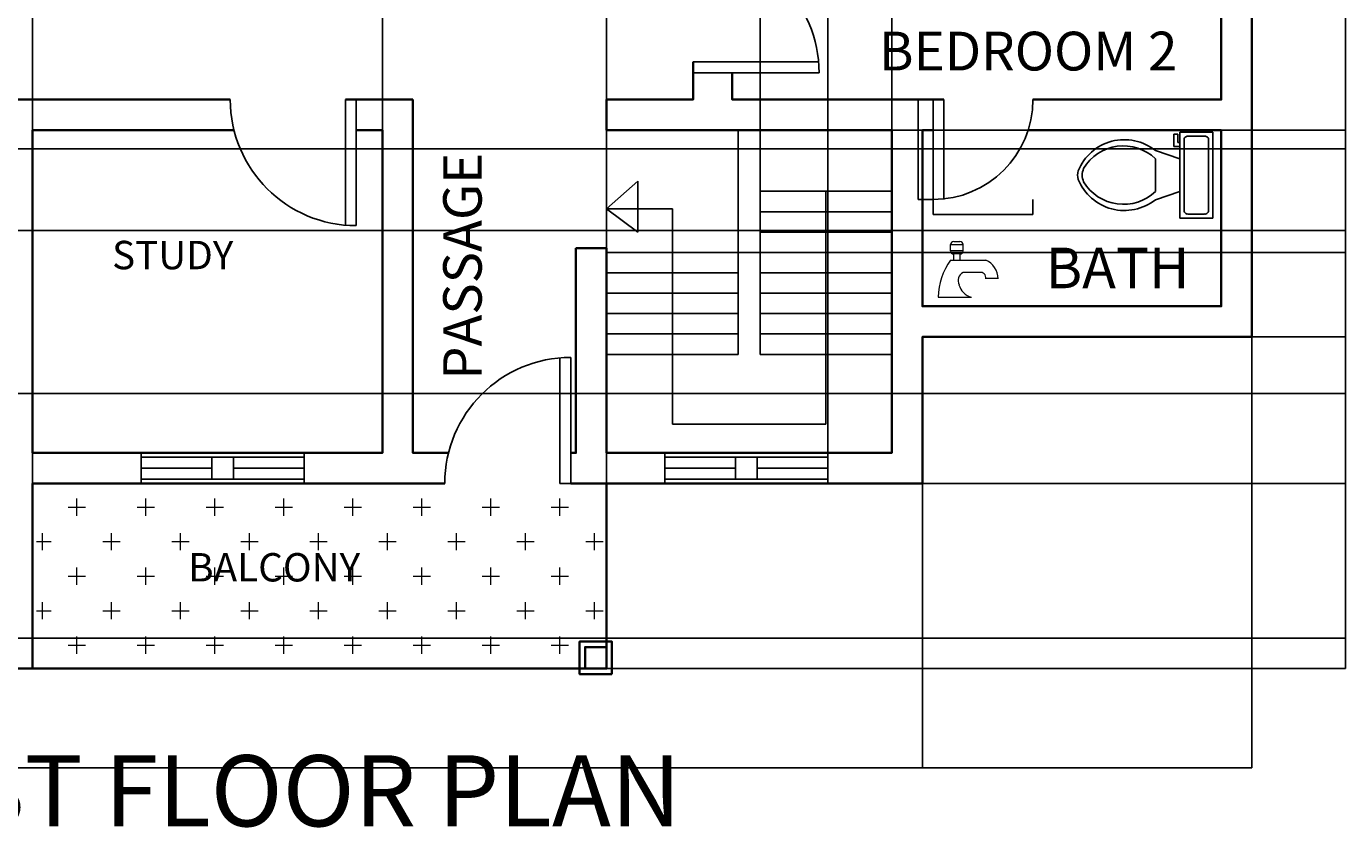
# Model space of a CAD drawing. Units: millimetres. Extents: x 19292 to 100733, y 12374 to 26974.
# Tile 20 of 24: x 47819 to 57530, y 12374 to 18270. Entities that reach past the tile are written whole.
import ezdxf

# ---------------------------------------------------------------- set-up
doc = ezdxf.new("R2010")
doc.units = ezdxf.units.MM
for name, color, linetype, lineweight in [('A-ANNO-DIMS', 2, 'Continuous', 18), ('A-ANNO-TEXT', 7, 'Continuous', 35), ('A-AREA-IDEN', 3, 'Continuous', 25), ('A-DOOR', 4, 'Continuous', 25), ('A-FLOR-FIXT', 9, 'Continuous', 18), ('A-FLOR-PATT', 252, 'Continuous', 13), ('A-FLOR-STRS', 1, 'Continuous', 25), ('A-GLAZ', 3, 'Continuous', 25), ('A-WALL', 7, 'Continuous', 35)]:
    doc.layers.add(name, color=color, linetype=linetype, lineweight=lineweight)
doc.layers.add('FURNITURE', color=40, linetype='Continuous')
doc.layers.add('WINDOWS', color=50, linetype='Continuous')
doc.styles.get("Standard").update_dxf_attribs({"font": 'arial.ttf'})
doc.dimstyles.get("Standard").update_dxf_attribs({"dimtxt": 0.18, "dimasz": 0.18, "dimexe": 0.18, "dimexo": 0.0625, "dimgap": 0.09, "dimtad": 0, "dimtih": 1, "dimtoh": 1, "dimdec": 4, "dimzin": 0, "dimdsep": 46, "dimtxsty": 'Standard', "dimcen": 0.09, "dimadec": 0, "dimazin": 0, "dimtfac": 1, "dimtdec": 4, "dimtofl": 0, "dimtmove": 0, "dimatfit": 3, "dimfxl": 1, "dimtolj": 1, "dimtzin": 0, "dimarcsym": 0})

# ---------------------------------------------------------------- blocks, each defined once
blk = doc.blocks.new('WW')
at = {"layer": 'WINDOWS'}
for p, q in [((-5183.9, -4940.9), (-3983.9, -4940.9)), ((-4663.9, -4940.9), (-4663.9, -5100.9)), ((-4503.9, -4940.9), (-4503.9, -5100.9)), ((-4503.9, -4940.9), (-4503.9, -5100.9)), ((-5183.9, -5020.9), (-4663.9, -5020.9)), ((-4503.9, -5020.9), (-3983.9, -5020.9)), ((-5183.9, -5100.9), (-3983.9, -5100.9))]:
    blk.add_line(p, q, dxfattribs=at)
for points in [[(-5183.9, -5133.4), (-5183.9, -4908.4)], [(-3983.9, -4908.4), (-3983.9, -5133.4)]]:
    blk.add_lwpolyline(points, dxfattribs=at)
blk = doc.blocks.new('WC01')
at = {"layer": 'FURNITURE'}
for p, q in [((10.5, 0), (-10.5, 0)), ((-10.5, 0), (-10.5, -8)), ((10.5, -8), (10.5, 0)), ((-9.5, -2), (-9.5, -6)), ((8.5, -1), (-8.5, -1)), ((9.5, -6), (9.5, -2)), ((-10.5, -8), (10.5, -8)), ((-10, -9.5), (-10, -8.5)), ((-10, -8.5), (-8, -8.5)), ((-7, -9.5), (-10, -9.5)), ((-8.5, -7), (8.5, -7)), ((-8, -8.5), (-8, -8)), ((-7, -8), (-7, -9.5)), ((-4, -8), (-6, -14)), ((4, -8), (6, -14)), ((4, -14), (-4, -14))]:
    blk.add_line(p, q, dxfattribs=at)
for centre, radius, start, end in [((-8.62, -1.88), 0.884, 81.8699, 188.1301), ((8.62, -1.88), 0.884, 351.8699, 98.1301), ((-8.62, -6.12), 0.884, 171.8699, 278.1301), ((8.62, -6.12), 0.884, 261.8699, 8.1301), ((3.52, -21.58), 12.17, 141.4691, 247.9714), ((4.2, -21.82), 11.33, 136.3677, 238.9468), ((-3.52, -21.58), 12.17, 292.0284, 38.5307), ((-4.2, -21.82), 11.33, 301.053, 43.6321), ((0, -27.88), 4, 245.7318, 294.2682), ((0, -29), 4, 254.8605, 285.1395)]:
    blk.add_arc(centre, radius, start, end, dxfattribs=at)
blk = doc.blocks.new('TAP-SIDELEV')
for p, q in [((1, 4.25), (2, 4.25)), ((2, 3.75), (1, 3.75)), ((1.25, 3), (1.25, 3.5)), ((1.75, 3.5), (1.75, 3)), ((1, 3), (3.84, 3)), ((3.53, 2), (2, 2)), ((4.84, 1.5), (3.84, 1.5)), ((0, 0), (0.25, 0)), ((0.25, 0), (2.68, 0))]:
    blk.add_line(p, q)
for points in [[(1.25, 4.5), (1.75, 4.5)], [(1, 3.75), (1, 4.25)], [(1.75, 3.5), (1.25, 3.5)], [(2, 4.25), (2, 3.75)]]:
    blk.add_lwpolyline(points)
for centre, radius, start, end in [((1.24, 4.26), 0.243, 88.2224, 181.7776), ((1.76, 4.26), 0.243, 358.2224, 91.7776), ((1.24, 3.74), 0.243, 178.2224, 271.7776), ((1.76, 3.74), 0.243, 268.2224, 1.7776), ((5.08, -0.03), 5.08, 143.4467, 179.6834), ((3.17, 1.47), 1.67, 0.9828, 66.4049), ((2.38, 1.33), 0.773, 119.1801, 204.8716), ((3.43, 1.59), 0.417, 347.0192, 102.9808), ((3.05, 1.38), 1.43, 195.2551, 254.7449)]:
    blk.add_arc(centre, radius, start, end)
blk = doc.blocks.new('DOOR-900')
for p, q in [((927.7, 80), (0, 80)), ((927.7, 0), (927.7, 80)), ((927.7, 0), (927.7, 80)), ((927.7, 0), (0, 0))]:
    blk.add_line(p, q)
blk.add_arc((927.7, 0), 927.7, 90, 180)
blk = doc.blocks.new('DOOR-SWING-900')
blk.add_line((927.7, 927.7), (927.7, 0))
blk.add_arc((927.7, 927.7), 927.7, 180, 270)
blk = doc.blocks.new('DOOR-SWING-750')
blk.add_line((0, 0), (735.3, 0))
blk.add_arc((0, 0), 735.3, 0, 90)
blk = doc.blocks.new('*D32')
at = {"layer": 'A-ANNO-DIMS', "color": 0, "lineweight": -2, "transparency": 16777216}
for p, q in [((54493.3, 16996.1), (54493.3, 16885.7)), ((55228.6, 16996.1), (55228.6, 16885.7)), ((54493.5, 16885.8), (54859.7, 16885.8)), ((55228.4, 16885.8), (54862.2, 16885.8))]:
    blk.add_line(p, q, dxfattribs=at)
at = {"layer": 'A-ANNO-DIMS', "color": 0, "transparency": 16777216}
for points in [[(54493.5, 16885.9), (54493.5, 16885.8), (54493.3, 16885.8)], [(55228.4, 16885.9), (55228.4, 16885.8), (55228.6, 16885.8)]]:
    blk.add_solid(points, dxfattribs=at)
at = {"layer": 'Defpoints', "color": 0, "transparency": 16777216}
for p in [(54493.3, 16996.1), (55228.6, 16996.1), (55228.6, 16885.8)]:
    blk.add_point(p, dxfattribs=at)
at = {"layer": 'A-ANNO-DIMS', "color": 0, "transparency": 16777216, "insert": (54860.9, 16885.8), "char_height": 0.18, "attachment_point": 5}
blk.add_mtext('\\A1;DOOR 750 735 TYP.', dxfattribs=at)
blk = doc.blocks.new('*D33')
at = {"layer": 'A-ANNO-DIMS', "color": 0, "lineweight": -2, "transparency": 16777216}
for p, q in [((54493.2, 17731.4), (54382.8, 17731.4)), ((54383, 17731.2), (54383, 17363.9)), ((54383, 16996.3), (54383, 17363.6)), ((54493.2, 16996.1), (54382.8, 16996.1))]:
    blk.add_line(p, q, dxfattribs=at)
at = {"layer": 'A-ANNO-DIMS', "color": 0, "transparency": 16777216}
for points in [[(54383, 17731.2), (54383, 17731.2), (54383, 17731.4)], [(54383, 16996.3), (54383, 16996.3), (54383, 16996.1)]]:
    blk.add_solid(points, dxfattribs=at)
at = {"layer": 'Defpoints', "color": 0, "transparency": 16777216}
for p in [(54493.3, 17731.4), (54383, 16996.1), (54493.3, 16996.1)]:
    blk.add_point(p, dxfattribs=at)
at = {"layer": 'A-ANNO-DIMS', "color": 0, "transparency": 16777216, "insert": (54383, 17363.8), "char_height": 0.18, "attachment_point": 5}
blk.add_mtext('\\A1;735 TYP.', dxfattribs=at)
blk = doc.blocks.new('*D103')
at = {"layer": 'A-ANNO-DIMS', "color": 0, "lineweight": -2, "transparency": 16777216}
for p, q in [((44268, 15569), (57530.2, 15569)), ((57530, 15568.8), (57530, 14669.2)), ((57530, 13769.2), (57530, 14668.8)), ((44268, 13769), (57530.2, 13769))]:
    blk.add_line(p, q, dxfattribs=at)
at = {"layer": 'A-ANNO-DIMS', "color": 0, "transparency": 16777216}
for points in [[(57530, 15568.8), (57530.1, 15568.8), (57530, 15569)], [(57530, 13769.2), (57530.1, 13769.2), (57530, 13769)]]:
    blk.add_solid(points, dxfattribs=at)
at = {"layer": 'Defpoints', "color": 0, "transparency": 16777216}
for p in [(44268, 15569), (57530, 15569), (44268, 13769)]:
    blk.add_point(p, dxfattribs=at)
at = {"layer": 'A-ANNO-DIMS', "color": 0, "transparency": 16777216, "insert": (57530, 14669), "char_height": 0.18, "attachment_point": 5}
blk.add_mtext('\\A1;1800', dxfattribs=at)
blk = doc.blocks.new('*D104')
at = {"layer": 'A-ANNO-DIMS', "color": 0, "lineweight": -2, "transparency": 16777216}
for p, q in [((44268, 17369), (57530.2, 17369)), ((57530, 17368.8), (57530, 17069.2)), ((57530, 16769.2), (57530, 17068.8)), ((44268, 16769), (57530.2, 16769))]:
    blk.add_line(p, q, dxfattribs=at)
at = {"layer": 'A-ANNO-DIMS', "color": 0, "transparency": 16777216}
for points in [[(57530, 17368.8), (57530.1, 17368.8), (57530, 17369)], [(57530, 16769.2), (57530.1, 16769.2), (57530, 16769)]]:
    blk.add_solid(points, dxfattribs=at)
at = {"layer": 'Defpoints', "color": 0, "transparency": 16777216}
for p in [(44268, 17369), (57530, 17369), (44268, 16769)]:
    blk.add_point(p, dxfattribs=at)
at = {"layer": 'A-ANNO-DIMS', "color": 0, "transparency": 16777216, "insert": (57530, 17069), "char_height": 0.18, "attachment_point": 5}
blk.add_mtext('\\A1;600', dxfattribs=at)
blk = doc.blocks.new('*D105')
at = {"layer": 'A-ANNO-DIMS', "color": 0, "lineweight": -2, "transparency": 16777216}
for p, q in [((54414.6, 14906.4), (57530.2, 14906.4)), ((57530, 14906.2), (57530, 14225.4)), ((57530, 13544.2), (57530, 14225)), ((52089.7, 13544), (57530.2, 13544))]:
    blk.add_line(p, q, dxfattribs=at)
at = {"layer": 'A-ANNO-DIMS', "color": 0, "transparency": 16777216}
for points in [[(57530, 14906.2), (57530.1, 14906.2), (57530, 14906.4)], [(57530, 13544.2), (57530.1, 13544.2), (57530, 13544)]]:
    blk.add_solid(points, dxfattribs=at)
at = {"layer": 'Defpoints', "color": 0, "transparency": 16777216}
for p in [(54414.5, 14906.4), (57530, 14906.4), (52089.7, 13544)]:
    blk.add_point(p, dxfattribs=at)
at = {"layer": 'A-ANNO-DIMS', "color": 0, "transparency": 16777216, "insert": (57530, 14225.2), "char_height": 0.18, "attachment_point": 5}
blk.add_mtext('\\A1;1362.4', dxfattribs=at)
blk = doc.blocks.new('*D106')
at = {"layer": 'A-ANNO-DIMS', "color": 0, "lineweight": -2, "transparency": 16777216}
for p, q in [((56840.1, 15985.7), (57530.2, 15985.7)), ((57530, 15985.5), (57530, 15446.2)), ((57530, 14906.6), (57530, 15445.9)), ((54414.6, 14906.4), (57530.2, 14906.4))]:
    blk.add_line(p, q, dxfattribs=at)
at = {"layer": 'A-ANNO-DIMS', "color": 0, "transparency": 16777216}
for points in [[(57530, 15985.5), (57530.1, 15985.5), (57530, 15985.7)], [(57530, 14906.6), (57530.1, 14906.6), (57530, 14906.4)]]:
    blk.add_solid(points, dxfattribs=at)
at = {"layer": 'Defpoints', "color": 0, "transparency": 16777216}
for p in [(56840, 15985.7), (57530, 15985.7), (54414.5, 14906.4)]:
    blk.add_point(p, dxfattribs=at)
at = {"layer": 'A-ANNO-DIMS', "color": 0, "transparency": 16777216, "insert": (57530, 15446.1), "char_height": 0.18, "attachment_point": 5}
blk.add_mtext('\\A1;1079.3', dxfattribs=at)
blk = doc.blocks.new('*D107')
at = {"layer": 'A-ANNO-DIMS', "color": 0, "lineweight": -2, "transparency": 16777216}
for p, q in [((56839.6, 19223.2), (57530.2, 19223.2)), ((57530, 19223), (57530, 17604.7)), ((57530, 15985.9), (57530, 17604.3)), ((56840.1, 15985.7), (57530.2, 15985.7))]:
    blk.add_line(p, q, dxfattribs=at)
at = {"layer": 'A-ANNO-DIMS', "color": 0, "transparency": 16777216}
for points in [[(57530, 19223), (57530.1, 19223), (57530, 19223.2)], [(57530, 15985.9), (57530.1, 15985.9), (57530, 15985.7)]]:
    blk.add_solid(points, dxfattribs=at)
at = {"layer": 'Defpoints', "color": 0, "transparency": 16777216}
for p in [(56839.5, 19223.2), (57530, 19223.2), (56840, 15985.7)]:
    blk.add_point(p, dxfattribs=at)
at = {"layer": 'A-ANNO-DIMS', "color": 0, "transparency": 16777216, "insert": (57530, 17604.5), "char_height": 0.18, "attachment_point": 5}
blk.add_mtext('\\A1;3237.5', dxfattribs=at)
blk = doc.blocks.new('*D112')
at = {"layer": 'A-ANNO-DIMS', "color": 0, "lineweight": -2, "transparency": 16777216}
for p, q in [((43389, 22860.7), (43389, 12813.8)), ((56840, 15985.7), (56840, 12813.8)), ((43389.2, 12814), (50114.1, 12814)), ((56839.9, 12814), (50114.9, 12814))]:
    blk.add_line(p, q, dxfattribs=at)
at = {"layer": 'A-ANNO-DIMS', "color": 0, "transparency": 16777216}
for points in [[(43389.2, 12814), (43389.2, 12814), (43389, 12814)], [(56839.9, 12814), (56839.9, 12814), (56840, 12814)]]:
    blk.add_solid(points, dxfattribs=at)
at = {"layer": 'Defpoints', "color": 0, "transparency": 16777216}
for p in [(43389, 22860.7), (56840, 15985.7), (56840, 12814)]:
    blk.add_point(p, dxfattribs=at)
at = {"layer": 'A-ANNO-DIMS', "color": 0, "transparency": 16777216, "insert": (50114.5, 12814), "char_height": 0.18, "attachment_point": 5}
blk.add_mtext('\\A1;13451', dxfattribs=at)
blk = doc.blocks.new('*D116')
at = {"layer": 'A-ANNO-DIMS', "color": 0, "lineweight": -2, "transparency": 16777216}
for p, q in [((47864.5, 13544.1), (47864.5, 23550.9)), ((47864.7, 23550.7), (49976.7, 23550.7)), ((52089.5, 23550.7), (49977.5, 23550.7)), ((52089.7, 13544.1), (52089.7, 23550.9))]:
    blk.add_line(p, q, dxfattribs=at)
at = {"layer": 'A-ANNO-DIMS', "color": 0, "transparency": 16777216}
for points in [[(47864.7, 23550.8), (47864.7, 23550.7), (47864.5, 23550.7)], [(52089.5, 23550.8), (52089.5, 23550.7), (52089.7, 23550.7)]]:
    blk.add_solid(points, dxfattribs=at)
at = {"layer": 'Defpoints', "color": 0, "transparency": 16777216}
for p in [(52089.7, 23550.7), (47864.5, 13544), (52089.7, 13544)]:
    blk.add_point(p, dxfattribs=at)
at = {"layer": 'A-ANNO-DIMS', "color": 0, "transparency": 16777216, "insert": (49977.1, 23550.7), "char_height": 0.18, "attachment_point": 5}
blk.add_mtext('\\A1;4225', dxfattribs=at)
blk = doc.blocks.new('*D117')
at = {"layer": 'A-ANNO-DIMS', "color": 0, "lineweight": -2, "transparency": 16777216}
for p, q in [((53718.5, 15131.5), (53718.5, 23550.9)), ((53718.6, 23550.7), (53953.6, 23550.7)), ((54189.3, 23550.7), (53954.4, 23550.7)), ((54189.5, 15131.5), (54189.5, 23550.9))]:
    blk.add_line(p, q, dxfattribs=at)
at = {"layer": 'A-ANNO-DIMS', "color": 0, "transparency": 16777216}
for points in [[(53718.6, 23550.8), (53718.6, 23550.7), (53718.5, 23550.7)], [(54189.3, 23550.8), (54189.3, 23550.7), (54189.5, 23550.7)]]:
    blk.add_solid(points, dxfattribs=at)
at = {"layer": 'Defpoints', "color": 0, "transparency": 16777216}
for p in [(54189.5, 23550.7), (53718.5, 15131.4), (54189.5, 15131.4)]:
    blk.add_point(p, dxfattribs=at)
at = {"layer": 'A-ANNO-DIMS', "color": 0, "transparency": 16777216, "insert": (53954, 23550.7), "char_height": 0.18, "attachment_point": 5}
blk.add_mtext('\\A1;471.1', dxfattribs=at)
blk = doc.blocks.new('*D118')
at = {"layer": 'A-ANNO-DIMS', "color": 0, "lineweight": -2, "transparency": 16777216}
for p, q in [((54414.519491, 15985.268979), (54414.519491, 12813.8126)), ((56840.042789, 15985.662601), (56840.042789, 12813.8126)), ((54414.699491, 12813.9926), (55626.815301, 12813.9926)), ((56839.862789, 12813.9926), (55627.746979, 12813.9926))]:
    blk.add_line(p, q, dxfattribs=at)
at = {"layer": 'A-ANNO-DIMS', "color": 0, "transparency": 16777216}
for points in [[(54414.699491, 12814.0226), (54414.699491, 12813.9626), (54414.519491, 12813.9926)], [(56839.862789, 12814.0226), (56839.862789, 12813.9626), (56840.042789, 12813.9926)]]:
    blk.add_solid(points, dxfattribs=at)
at = {"layer": 'Defpoints', "color": 0, "transparency": 16777216}
for p in [(54414.519491, 15985.331479), (56840.042789, 15985.725101), (56840.042789, 12813.9926)]:
    blk.add_point(p, dxfattribs=at)
at = {"layer": 'A-ANNO-DIMS', "color": 0, "transparency": 16777216, "insert": (55627.28114, 12813.9926), "char_height": 0.18, "attachment_point": 5}
blk.add_mtext('\\A1;2425.5', dxfattribs=at)
blk = doc.blocks.new('*D119')
at = {"layer": 'A-ANNO-DIMS', "color": 0, "lineweight": -2, "transparency": 16777216}
for p, q in [((47864.5, 15131.5), (47864.5, 23550.9)), ((47864.7, 23550.7), (49151.7, 23550.7)), ((50439.3, 23550.7), (49152.4, 23550.7)), ((50439.5, 15131.5), (50439.5, 23550.9))]:
    blk.add_line(p, q, dxfattribs=at)
at = {"layer": 'A-ANNO-DIMS', "color": 0, "transparency": 16777216}
for points in [[(47864.7, 23550.8), (47864.7, 23550.7), (47864.5, 23550.7)], [(50439.3, 23550.8), (50439.3, 23550.7), (50439.5, 23550.7)]]:
    blk.add_solid(points, dxfattribs=at)
at = {"layer": 'Defpoints', "color": 0, "transparency": 16777216}
for p in [(50439.5, 23550.7), (47864.5, 15131.4), (50439.5, 15131.4)]:
    blk.add_point(p, dxfattribs=at)
at = {"layer": 'A-ANNO-DIMS', "color": 0, "transparency": 16777216, "insert": (49152, 23550.7), "char_height": 0.18, "attachment_point": 5}
blk.add_mtext('\\A1;2575', dxfattribs=at)
blk = doc.blocks.new('*D120')
at = {"layer": 'A-ANNO-DIMS', "color": 0, "lineweight": -2, "transparency": 16777216}
for p, q in [((53219.5, 17056.5), (53219.5, 23550.9)), ((53219.7, 23550.7), (53704.2, 23550.7)), ((54189.3, 23550.7), (53704.8, 23550.7)), ((54189.5, 17056.5), (54189.5, 23550.9))]:
    blk.add_line(p, q, dxfattribs=at)
at = {"layer": 'A-ANNO-DIMS', "color": 0, "transparency": 16777216}
for points in [[(53219.7, 23550.8), (53219.7, 23550.7), (53219.5, 23550.7)], [(54189.3, 23550.8), (54189.3, 23550.7), (54189.5, 23550.7)]]:
    blk.add_solid(points, dxfattribs=at)
at = {"layer": 'Defpoints', "color": 0, "transparency": 16777216}
for p in [(54189.5, 23550.7), (53219.5, 17056.4), (54189.5, 17056.4)]:
    blk.add_point(p, dxfattribs=at)
at = {"layer": 'A-ANNO-DIMS', "color": 0, "transparency": 16777216, "insert": (53704.5, 23550.7), "char_height": 0.18, "attachment_point": 5}
blk.add_mtext('\\A1;970', dxfattribs=at)
blk = doc.blocks.new('*D121')
at = {"layer": 'A-ANNO-DIMS', "color": 0, "lineweight": -2, "transparency": 16777216}
for p, q in [((52089.6, 17506.4), (57530.2, 17506.4)), ((57530, 17506.2), (57530, 17056.6)), ((57530, 16606.6), (57530, 17056.2)), ((52089.6, 16606.4), (57530.2, 16606.4))]:
    blk.add_line(p, q, dxfattribs=at)
at = {"layer": 'A-ANNO-DIMS', "color": 0, "transparency": 16777216}
for points in [[(57530, 17506.2), (57530.1, 17506.2), (57530, 17506.4)], [(57530, 16606.6), (57530.1, 16606.6), (57530, 16606.4)]]:
    blk.add_solid(points, dxfattribs=at)
at = {"layer": 'Defpoints', "color": 0, "transparency": 16777216}
for p in [(52089.5, 17506.4), (52089.5, 16606.4), (57530, 16606.4)]:
    blk.add_point(p, dxfattribs=at)
at = {"layer": 'A-ANNO-DIMS', "color": 0, "transparency": 16777216, "insert": (57530, 17056.4), "char_height": 0.18, "attachment_point": 5}
blk.add_mtext('\\A1;900', dxfattribs=at)

msp = doc.modelspace()

# ---------------------------------------------------------------- hatches: boundary and pattern name
at = {"layer": 'A-FLOR-PATT'}
h = msp.add_hatch(dxfattribs=at)
h.set_pattern_fill('CROSS', color=256, scale=40)
h.set_pattern_definition([(0, (20694.86, 0), (254, 254), [127, -381]), (90, (20758.36, -63.5), (-254, 254), [127, -381])])
h.paths.add_polyline_path([(52089.658, 14906.403), (51746.401, 14906.403), (50163.431, 14906.403), (47893.674, 14906.403), (47893.674, 13543.993), (52089.658, 13543.993)])
h.paths.add_polyline_path([(48522.956, 14036.581), (51324.024, 14036.581), (51324.024, 14443.478), (48522.956, 14443.478)], flags=24)

# ---------------------------------------------------------------- linework, layer by layer
at = {"layer": 'A-DOOR'}
for p, q in [((52726.51, 18008.189), (53654.209, 18008.189)), ((50167.674, 17731.403), (50167.674, 16803.704)), ((50247.674, 17731.403), (50247.674, 16803.704)), ((50247.674, 17731.403), (50247.674, 16803.704)), ((54573.302, 17731.403), (54573.302, 16996.131))]:
    msp.add_line(p, q, dxfattribs=at)
msp.add_arc((50247.674, 17731.403), 927.699, 180, 270, dxfattribs=at)
at = {"layer": 'A-FLOR-STRS'}
for p, q in [((52089.519, 17506.403), (53059.519, 17506.403)), ((53059.519, 17506.403), (53059.519, 15856.403)), ((52089.519, 16927.763), (52320.043, 17131.846)), ((52320.043, 17131.846), (52320.043, 16756.403)), ((53219.519, 17056.403), (53219.519, 15856.403)), ((53219.519, 17056.403), (54189.519, 17056.403)), ((53704.519, 17056.403), (53704.519, 15343.431)), ((52574.519, 16927.763), (52089.519, 16927.763)), ((52320.043, 16756.403), (52089.519, 16927.763)), ((52574.519, 15343.431), (52574.519, 16927.763)), ((53219.519, 16906.403), (54189.519, 16906.403)), ((53219.519, 16756.403), (54189.519, 16756.403)), ((52089.519, 16606.403), (53059.519, 16606.403)), ((53219.519, 16606.403), (54189.519, 16606.403)), ((52089.519, 16456.403), (53059.519, 16456.403)), ((53219.519, 16456.403), (54189.519, 16456.403)), ((52089.519, 16306.403), (53059.519, 16306.403)), ((53219.519, 16306.403), (54189.519, 16306.403)), ((52089.519, 16156.403), (53059.519, 16156.403)), ((53219.519, 16156.403), (54189.519, 16156.403)), ((52089.519, 16006.403), (53059.519, 16006.403)), ((53219.519, 16006.403), (54189.519, 16006.403)), ((52089.519, 15856.403), (53059.519, 15856.403)), ((53219.519, 15856.403), (54189.519, 15856.403)), ((53704.519, 15343.431), (52574.519, 15343.431))]:
    msp.add_line(p, q, dxfattribs=at)
at = {"layer": 'A-WALL'}
for p, q in [((52089.519, 17506.403), (52089.519, 17731.403)), ((51864.519, 16638.191), (52089.519, 16638.191))]:
    msp.add_line(p, q, dxfattribs=at)
for points in [[(43388.992, 22860.725), (49063.992, 22860.725), (49063.992, 22460.725), (56838.992, 22460.725), (56840.043, 15985.725), (54414.519, 15985.331), (54414.519, 14906.403), (52089.658, 14906.403), (52089.658, 13543.993), (44043.674, 13543.993), (44026.778, 19012.695), (43388.992, 19010.725), (43388.992, 22860.725)], [(53014.796, 18809.957), (53014.796, 20981.403), (56614.796, 20981.403), (56614.796, 17731.403), (55228.574, 17731.403)], [(52726.51, 18008.189), (52726.51, 17731.403), (52089.519, 17731.403)], [(54573.302, 17731.403), (53014.796, 17731.403), (53014.796, 17928.189)], [(49319.975, 17731.403), (47667.98, 17731.403), (47667.98, 17593.993), (47552.886, 17593.993)], [(50664.519, 17731.403), (50167.674, 17731.403)], [(50926.401, 15131.403), (50664.519, 15131.403), (50664.519, 17731.403)], [(50247.674, 17506.403), (50439.519, 17506.403), (50439.519, 15131.403), (47864.519, 15131.403), (47864.519, 17506.403), (49347.674, 17506.403)], [(54189.519, 17506.403), (52089.519, 17506.403)], [(52089.519, 16638.191), (52089.519, 15131.403), (54189.519, 15131.403), (54189.519, 17506.403), (53838.853, 17506.403)], [(55193.302, 17506.403), (56615.006, 17506.403), (56615.006, 16210.689), (54414.519, 16210.689), (54414.519, 17506.403), (54493.302, 17506.403)], [(51864.519, 16638.191), (51864.519, 15131.403), (51826.401, 15131.403)], [(51826.401, 14906.403), (52089.658, 14906.403), (52089.658, 13543.993), (47864.519, 13543.993), (47864.519, 14906.403), (50898.703, 14906.403)]]:
    msp.add_lwpolyline(points, dxfattribs=at)
for points in [[(52129.658, 13503.993), (51891.206, 13503.993), (51891.206, 13742.444), (52129.658, 13742.444)], [(52089.658, 13543.993), (51931.206, 13543.993), (51931.206, 13702.444), (52089.658, 13702.444)]]:
    msp.add_lwpolyline(points, close=True, dxfattribs=at)

# ---------------------------------------------------------------- block references
at = {"layer": 'A-DOOR', "extrusion": (0, 0, -1), "zscale": -1}
for name, p, rotation in [('DOOR-SWING-900', (-53654.209, 18855.887), 269.9999999999991), ('DOOR-900', (-51826.401, 15834.102), 270.0000000000001)]:
    msp.add_blockref(name, p, dxfattribs=dict(at, rotation=rotation))
at = {"layer": 'A-DOOR', "rotation": 269.9999999999999}
msp.add_blockref('DOOR-SWING-750', (54493.302, 17731.404), dxfattribs=at)
at = {"layer": 'A-FLOR-FIXT', "xscale": 30.13269765108242, "yscale": 30.13269765108242, "zscale": 30.13269765108242, "rotation": 270}
msp.add_blockref('WC01', (56551.959, 17175.736), dxfattribs=at)
at = {"layer": 'A-FLOR-FIXT', "xscale": 91.03318940714036, "yscale": 91.03318940714036, "zscale": 91.03318940714036}
msp.add_blockref('TAP-SIDELEV', (54531.677, 16277.132), dxfattribs=at)
at = {"layer": 'A-GLAZ'}
for p in [(53848.457, 20039.78), (57702.325, 20039.78)]:
    msp.add_blockref('WW', p, dxfattribs=at)

# ---------------------------------------------------------------- texts
at = {"layer": 'A-ANNO-TEXT'}
msp.add_text('FIRST FLOOR PLAN', height=523.26848, dxfattribs=at).set_placement((46324.602, 12383.031))
at = {"layer": 'A-AREA-IDEN'}
for s, height, p in [('BEDROOM 2', 285.4899, (54094.143, 17945.752)), ('STUDY', 208.8711, (48449.531, 16482.903)), ('BATH', 299.1707, (55322.833, 16343.05)), ('BALCONY', 208.8711, (49010.064, 14185.033))]:
    msp.add_text(s, height=height, dxfattribs=at).set_placement(p)
msp.add_text('PASSAGE', height=283.3894, rotation=90, dxfattribs=at).set_placement((51170.564, 15669.45))

# ---------------------------------------------------------------- dimensions: what is measured, and where the dimension line sits
at = {"layer": 'A-ANNO-DIMS'}
for base, p1, p2, override, picture, middle in [((52089.658, 23550.725), (47864.519, 13543.993), (52089.658, 13543.993), {"dimdec": 0, "dimlfac": 1, "dimrnd": 0, "dimzin": 0, "dimdsep": 46, "dimlunit": 2}, '*D116', (49977.089, 23550.725)), ((50439.519, 23550.725), (47864.519, 15131.403), (50439.519, 15131.403), {"dimdec": 0, "dimlfac": 1, "dimrnd": 0, "dimzin": 0, "dimdsep": 46, "dimlunit": 2}, '*D119', (49152.019, 23550.725)), ((54189.519, 23550.725), (53219.519, 17056.403), (54189.519, 17056.403), {"dimdec": 0, "dimlfac": 1, "dimrnd": 0, "dimzin": 0, "dimdsep": 46, "dimlunit": 2}, '*D120', (53704.519, 23550.725)), ((54189.519, 23550.725), (53718.457, 15131.403), (54189.519, 15131.403), {"dimdec": 1, "dimlfac": 1, "dimrnd": 0, "dimzin": 0, "dimdsep": 46, "dimlunit": 2}, '*D117', (53953.988, 23550.725)), ((56840.043, 12813.993), (43388.992, 22860.725), (56840.043, 15985.725), {"dimdec": 0, "dimlfac": 1, "dimrnd": 0, "dimzin": 0, "dimdsep": 46, "dimlunit": 2}, '*D112', (50114.517, 12813.993)), ((56840.043, 12813.993), (54414.519, 15985.331), (56840.043, 15985.725), {"dimdec": 1, "dimlfac": 1, "dimrnd": 0, "dimzin": 0, "dimdsep": 46, "dimlunit": 2}, '*D118', (55627.281, 12813.993))]:
    dim = msp.add_linear_dim(base=base, p1=p1, p2=p2, dimstyle='Standard', override=override, dxfattribs=at)
    dim.commit()
    dim.dimension.update_dxf_attribs({"geometry": picture, "text_midpoint": middle})
for base, p1, p2, override, picture, middle in [((57530.043, 19223.225), (56840.043, 15985.725), (56839.517, 19223.225), {"dimdec": 1, "dimlfac": 1, "dimrnd": 0, "dimzin": 0, "dimdsep": 46, "dimlunit": 2}, '*D107', (57530.043, 17604.475)), ((57530.043, 16606.403), (52089.519, 17506.403), (52089.519, 16606.403), {"dimdec": 0, "dimlfac": 1, "dimrnd": 0, "dimzin": 0, "dimdsep": 46, "dimlunit": 2}, '*D121', (57530.043, 17056.403)), ((57530.043, 17368.993), (44267.98, 16768.993), (44267.98, 17368.993), {"dimdec": 0, "dimlfac": 1, "dimrnd": 0, "dimzin": 0, "dimdsep": 46, "dimlunit": 2}, '*D104', (57530.043, 17068.993)), ((57530.043, 15985.725), (54414.519, 14906.403), (56840.043, 15985.725), {"dimdec": 1, "dimlfac": 1, "dimrnd": 0, "dimzin": 0, "dimdsep": 46, "dimlunit": 2}, '*D106', (57530.043, 15446.064)), ((57530.043, 15568.993), (44267.98, 13768.993), (44267.98, 15568.993), {"dimdec": 0, "dimlfac": 1, "dimrnd": 0, "dimzin": 0, "dimdsep": 46, "dimlunit": 2}, '*D103', (57530.043, 14668.993)), ((57530.043, 14906.403), (52089.658, 13543.993), (54414.519, 14906.403), {"dimdec": 1, "dimlfac": 1, "dimrnd": 0, "dimzin": 0, "dimdsep": 46, "dimlunit": 2}, '*D105', (57530.043, 14225.198))]:
    dim = msp.add_linear_dim(base=base, p1=p1, p2=p2, angle=90, dimstyle='Standard', override=override, dxfattribs=at)
    dim.commit()
    dim.dimension.update_dxf_attribs({"geometry": picture, "text_midpoint": middle})
dim = msp.add_linear_dim(base=(54383.011, 16996.131), p1=(54493.302, 17731.403), p2=(54493.302, 16996.131), angle=270, text='<> TYP.', dimstyle='Standard', override={"dimdec": 0, "dimrnd": 0, "dimzin": 0, "dimlunit": 2}, dxfattribs=at)
dim.commit()
dim.dimension.update_dxf_attribs({"geometry": '*D33', "text_midpoint": (54383.011, 17363.767)})
dim = msp.add_linear_dim(base=(55228.574, 16885.84), p1=(54493.302, 16996.131), p2=(55228.574, 16996.131), text='DOOR 750 <> TYP.', dimstyle='Standard', override={"dimdec": 0, "dimrnd": 0, "dimzin": 0, "dimlunit": 2}, dxfattribs=at)
dim.commit()
dim.dimension.update_dxf_attribs({"geometry": '*D32', "text_midpoint": (54860.938, 16885.84)})

doc.saveas('drawing.dxf')
